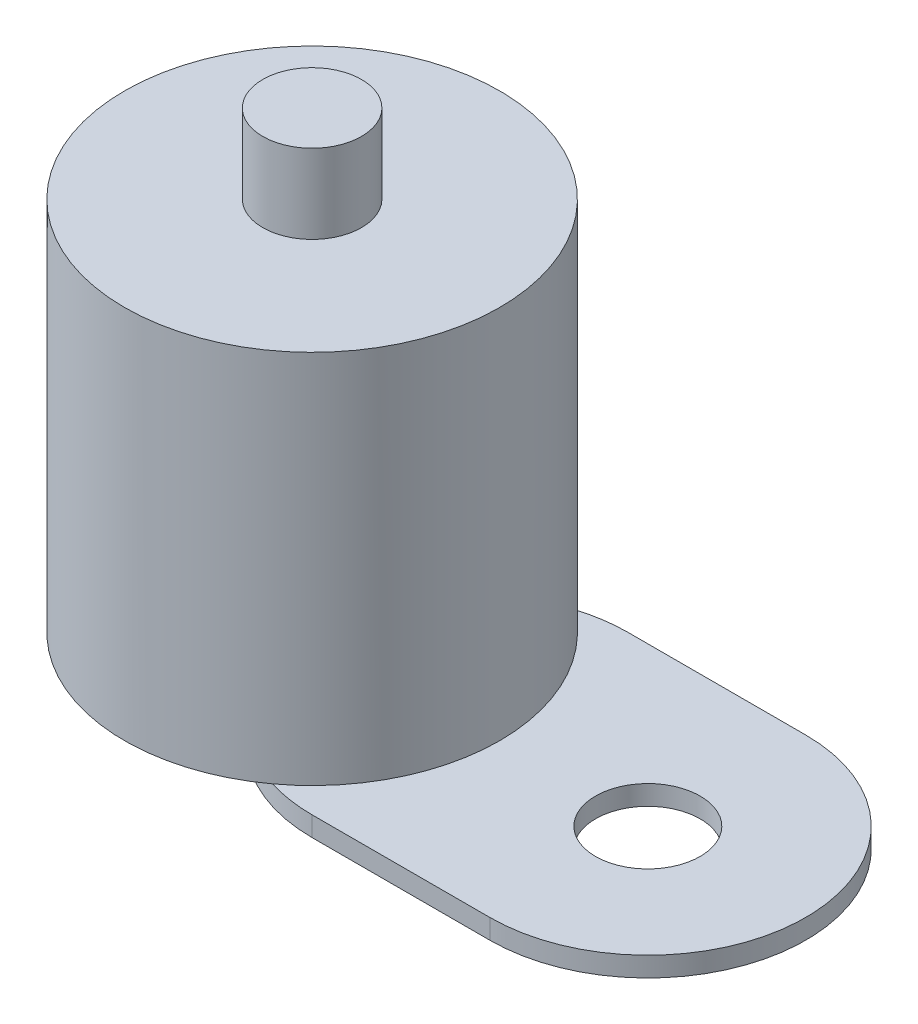
from build123d import *

# Parameters (mm, degrees)
MOUNTING_TAB_PROFILE_R               = 2.65
MOUNTING_TAB_1MM_WITH_HOLE_5_3_DEPTH = 1
CHAMBER_BODY_PROFILE_19_R            = 9.5
CHAMBER_BODY_19X19_DEPTH             = 19
TOP_PIN_PROFILE_5_R                  = 2.5
TOP_PIN_5X4_DEPTH                    = 4


with BuildPart() as part:
    # Mounting Tab Profile → Mounting Tab 1mm with Hole Ø5.3 (new body)
    with BuildSketch(Plane(origin=(0, 0, 0), x_dir=(1, 0, 0), z_dir=(0, 1, 0))):
        with BuildLine():
            Line((-4.5, 8), (4.5, 8))
            ThreePointArc((4.5, 8), (12.5, 0), (4.5, -8))
            Line((4.5, -8), (-4.5, -8))
            ThreePointArc((-4.5, -8), (-12.5, 0), (-4.5, 8))
        make_face()
        with Locations(Location((4.5, 0, 0), (0, 0, 270))):
            Circle(MOUNTING_TAB_PROFILE_R, mode=Mode.SUBTRACT)
    extrude(amount=MOUNTING_TAB_1MM_WITH_HOLE_5_3_DEPTH)

    # Chamber Body Profile Ø19 → Chamber Body Ø19x19 (add)
    with BuildSketch(Plane(origin=(0, 1, 0), x_dir=(1, 0, 0), z_dir=(0, 1, 0))):
        with Locations(Location((-12.5, 0, 0), (0, 0, 53.576426358))):
            Circle(CHAMBER_BODY_PROFILE_19_R)
    extrude(amount=CHAMBER_BODY_19X19_DEPTH)

    # Top Pin Profile Ø5 → Top Pin Ø5x4 (add)
    with BuildSketch(Plane(origin=(0, 20, 0), x_dir=(1, 0, 0), z_dir=(0, 1, 0))):
        with Locations(Location((-12.5, 0, 0), (0, 0, 270))):
            Circle(TOP_PIN_PROFILE_5_R)
    extrude(amount=TOP_PIN_5X4_DEPTH)


solid = part.part
